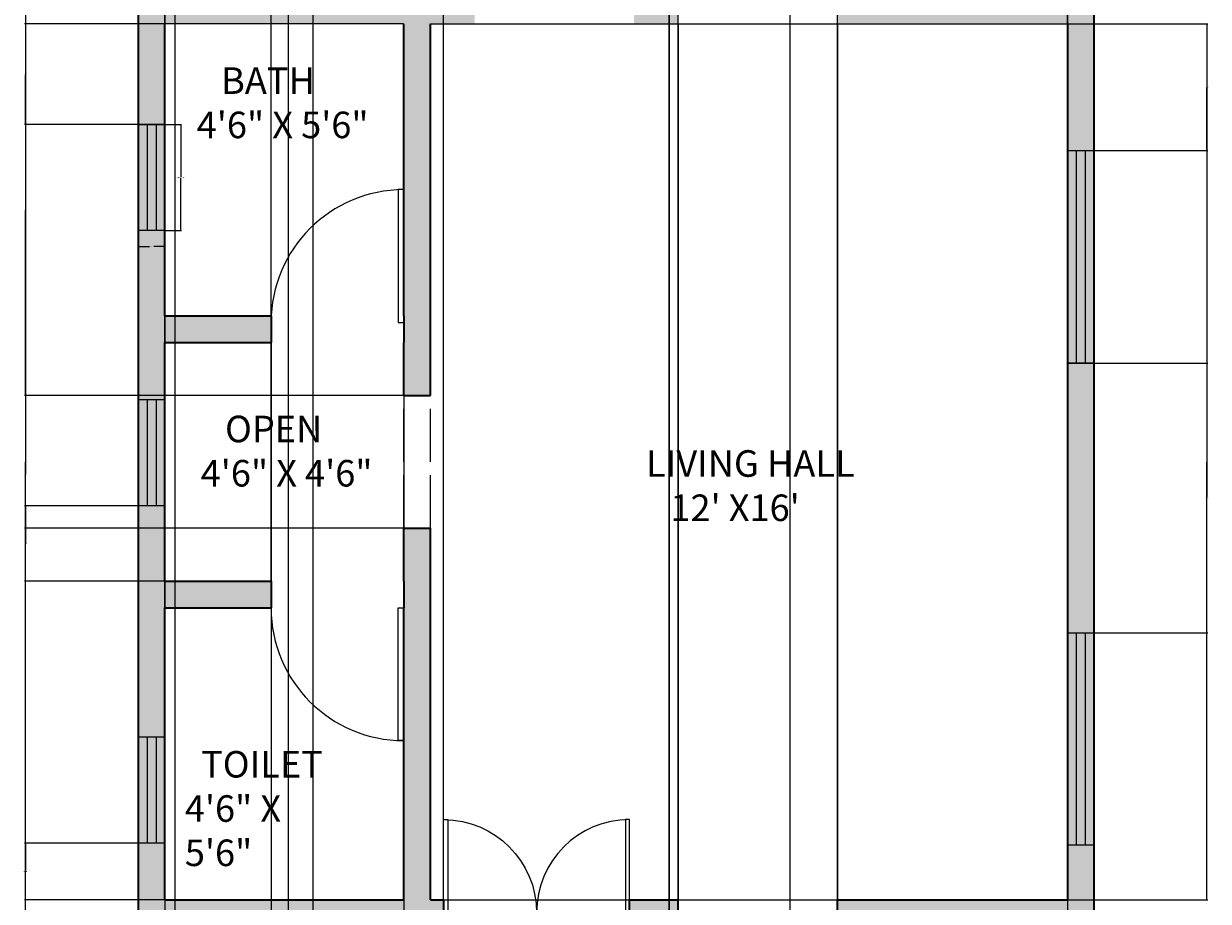
# Model space of a CAD drawing. Units: feet. Extents: x 4596233 to 4596501, y 5666486 to 5667044.
# Tile 2 of 3: x 4596233 to 4596501, y 5666688 to 5666886. Entities that reach past the tile are written whole.
import ezdxf

# ---------------------------------------------------------------- set-up
doc = ezdxf.new("R2010")
doc.units = ezdxf.units.FT
doc.linetypes.add('ACAD_ISO02W100', pattern=[15, 12, -3])
for name, color, linetype, lineweight in [('A-ANNO-DIMS', 2, 'Continuous', 18), ('A-DOOR-OVHD', 240, 'ACAD_ISO02W100', 18), ('A-WALL', 7, 'Continuous', 35), ('ANNOTATION', 170, 'Continuous', 18), ('DOOR', 240, 'Continuous', 18)]:
    doc.layers.add(name, color=color, linetype=linetype, lineweight=lineweight)
doc.layers.add('A-GLAZ', color=2, linetype='Continuous', lineweight=18, true_color=0xf1eb1f)
doc.layers.add('A-WALL-PATT', color=251, linetype='Continuous', lineweight=13, true_color=0x636466)
doc.styles.get("Standard").update_dxf_attribs({"font": 'arial.ttf'})
doc.dimstyles.get("Standard").update_dxf_attribs({"dimtxt": 0.18, "dimasz": 0.18, "dimexe": 0.18, "dimexo": 0.0625, "dimgap": 0.09, "dimtad": 0, "dimtih": 1, "dimtoh": 1, "dimdec": 0, "dimzin": 0, "dimdsep": 46, "dimlunit": 3, "dimtxsty": 'Standard', "dimcen": 0.09, "dimadec": 0, "dimazin": 0, "dimtfac": 1, "dimtdec": 0, "dimtofl": 0, "dimtmove": 0, "dimatfit": 3, "dimfxl": 1, "dimtolj": 1, "dimtzin": 0, "dimarcsym": 0})

# ---------------------------------------------------------------- blocks, each defined once
blk = doc.blocks.new('*U3')
for p, q in [((0, 0), (0, -6)), ((-40, 0), (-40, -6))]:
    blk.add_line(p, q)
blk.add_lwpolyline([(0, 0), (0, 40), (-1.75, 40), (-1.75, 0)], close=True)
blk.add_arc((0, 0), 40, 90, 180)
blk = doc.blocks.new('*U2')
for p, q in [((-40, 0), (-40, 6)), ((0, 0), (0, 6))]:
    blk.add_line(p, q)
blk.add_lwpolyline([(0, 0), (0, -40), (-1.75, -40), (-1.75, 0)], close=True)
blk.add_arc((0, 0), 40, 180, 270)
blk = doc.blocks.new('WIN-48IN')
h = blk.add_hatch(color=256)
h.dxf.hatch_style = 1
h.paths.add_polyline_path([(48, 2), (48, 4), (0, 4), (0, 2)])
for p, q in [((0, 6), (48, 6)), ((0, 0), (0, 6)), ((48, 6), (48, 0)), ((0, 4), (48, 4)), ((0, 2), (48, 2)), ((48, 0), (0, 0))]:
    blk.add_line(p, q)
blk = doc.blocks.new('WIN-24IN')
h = blk.add_hatch(color=256)
h.dxf.hatch_style = 1
h.paths.add_polyline_path([(2, 0), (4, 0), (4, 24), (2, 24)])
for p, q in [((0, 0), (0, 24)), ((0, 24), (6, 24)), ((2, 24), (2, 0)), ((4, 24), (4, 0)), ((6, 24), (6, 0)), ((6, 0), (0, 0))]:
    blk.add_line(p, q)
blk = doc.blocks.new('*D9')
at = {"layer": 'A-ANNO-DIMS', "color": 0, "lineweight": -2, "transparency": 16777216}
for p, q in [((4596264.91, 5666863.39), (4596268.63, 5666863.39)), ((4596268.45, 5666863.21), (4596268.45, 5666851.57)), ((4596268.45, 5666839.57), (4596268.45, 5666851.21)), ((4596264.91, 5666839.39), (4596268.63, 5666839.39))]:
    blk.add_line(p, q, dxfattribs=at)
at = {"layer": 'A-ANNO-DIMS', "color": 0, "transparency": 16777216}
for points in [[(4596268.42, 5666863.21), (4596268.48, 5666863.21), (4596268.45, 5666863.39)], [(4596268.42, 5666839.57), (4596268.48, 5666839.57), (4596268.45, 5666839.39)]]:
    blk.add_solid(points, dxfattribs=at)
at = {"layer": 'Defpoints', "color": 0, "transparency": 16777216}
for p in [(4596264.85, 5666863.39), (4596268.45, 5666863.39), (4596264.85, 5666839.39)]:
    blk.add_point(p, dxfattribs=at)
at = {"layer": 'A-ANNO-DIMS', "color": 0, "transparency": 16777216, "insert": (4596268.45, 5666851.39), "char_height": 0.18, "attachment_point": 5}
blk.add_mtext('\\A1;WINDOW 24 TYP.', dxfattribs=at)
blk = doc.blocks.new('*D10')
at = {"layer": 'A-ANNO-DIMS', "color": 0, "lineweight": -2, "transparency": 16777216}
for p, q in [((4596258.85, 5666839.33), (4596258.85, 5666835.61)), ((4596264.85, 5666839.33), (4596264.85, 5666835.61)), ((4596259.03, 5666835.79), (4596261.39, 5666835.79)), ((4596264.67, 5666835.79), (4596262.31, 5666835.79))]:
    blk.add_line(p, q, dxfattribs=at)
at = {"layer": 'A-ANNO-DIMS', "color": 0, "transparency": 16777216}
for points in [[(4596259.03, 5666835.82), (4596259.03, 5666835.76), (4596258.85, 5666835.79)], [(4596264.67, 5666835.82), (4596264.67, 5666835.76), (4596264.85, 5666835.79)]]:
    blk.add_solid(points, dxfattribs=at)
at = {"layer": 'Defpoints', "color": 0, "transparency": 16777216}
for p in [(4596258.85, 5666839.39), (4596264.85, 5666839.39), (4596264.85, 5666835.79)]:
    blk.add_point(p, dxfattribs=at)
at = {"layer": 'A-ANNO-DIMS', "color": 0, "transparency": 16777216, "insert": (4596261.85, 5666835.79), "char_height": 0.18, "attachment_point": 5}
blk.add_mtext('\\A1;6 TYP.', dxfattribs=at)
blk = doc.blocks.new('*D12')
at = {"layer": 'A-ANNO-DIMS', "color": 0, "lineweight": -2, "transparency": 16777216}
for p, q in [((4596258.79, 5667018.15), (4596233.12, 5667018.15)), ((4596233.3, 5667017.97), (4596233.3, 5666784.33)), ((4596233.3, 5666550.33), (4596233.3, 5666783.97)), ((4596258.79, 5666550.15), (4596233.12, 5666550.15))]:
    blk.add_line(p, q, dxfattribs=at)
at = {"layer": 'A-ANNO-DIMS', "color": 0, "transparency": 16777216}
for points in [[(4596233.27, 5667017.97), (4596233.33, 5667017.97), (4596233.3, 5667018.15)], [(4596233.27, 5666550.33), (4596233.33, 5666550.33), (4596233.3, 5666550.15)]]:
    blk.add_solid(points, dxfattribs=at)
at = {"layer": 'Defpoints', "color": 0, "transparency": 16777216}
for p in [(4596233.3, 5667018.15), (4596258.85, 5667018.15), (4596258.85, 5666550.15)]:
    blk.add_point(p, dxfattribs=at)
at = {"layer": 'A-ANNO-DIMS', "color": 0, "transparency": 16777216, "insert": (4596233.3, 5666784.15), "char_height": 0.18, "attachment_point": 5}
blk.add_mtext('\\A1;468', dxfattribs=at)
blk = doc.blocks.new('*D14')
at = {"layer": 'A-ANNO-DIMS', "color": 0, "lineweight": -2, "transparency": 16777216}
for p, q in [((4596324.91, 5666886.15), (4596500.58, 5666886.15)), ((4596500.4, 5666885.97), (4596500.4, 5666787.33)), ((4596500.4, 5666688.33), (4596500.4, 5666786.97)), ((4596324.91, 5666688.15), (4596500.58, 5666688.15))]:
    blk.add_line(p, q, dxfattribs=at)
at = {"layer": 'A-ANNO-DIMS', "color": 0, "transparency": 16777216}
for points in [[(4596500.37, 5666885.97), (4596500.43, 5666885.97), (4596500.4, 5666886.15)], [(4596500.37, 5666688.33), (4596500.43, 5666688.33), (4596500.4, 5666688.15)]]:
    blk.add_solid(points, dxfattribs=at)
at = {"layer": 'Defpoints', "color": 0, "transparency": 16777216}
for p in [(4596324.85, 5666886.15), (4596500.4, 5666886.15), (4596324.85, 5666688.15)]:
    blk.add_point(p, dxfattribs=at)
at = {"layer": 'A-ANNO-DIMS', "color": 0, "transparency": 16777216, "insert": (4596500.4, 5666787.15), "char_height": 0.18, "attachment_point": 5}
blk.add_mtext('\\A1;198', dxfattribs=at)
blk = doc.blocks.new('*D15')
at = {"layer": 'A-ANNO-DIMS', "color": 0, "lineweight": -2, "transparency": 16777216}
for p, q in [((4596378.85, 5666964.09), (4596378.85, 5666485.84)), ((4596468.85, 5666964.09), (4596468.85, 5666485.84)), ((4596379.03, 5666486.02), (4596423.63, 5666486.02)), ((4596468.67, 5666486.02), (4596424.07, 5666486.02))]:
    blk.add_line(p, q, dxfattribs=at)
at = {"layer": 'A-ANNO-DIMS', "color": 0, "transparency": 16777216}
for points in [[(4596379.03, 5666486.05), (4596379.03, 5666485.99), (4596378.85, 5666486.02)], [(4596468.67, 5666486.05), (4596468.67, 5666485.99), (4596468.85, 5666486.02)]]:
    blk.add_solid(points, dxfattribs=at)
at = {"layer": 'Defpoints', "color": 0, "transparency": 16777216}
for p in [(4596378.85, 5666964.15), (4596468.85, 5666964.15), (4596468.85, 5666486.02)]:
    blk.add_point(p, dxfattribs=at)
at = {"layer": 'A-ANNO-DIMS', "color": 0, "transparency": 16777216, "insert": (4596423.85, 5666486.02), "char_height": 0.18, "attachment_point": 5}
blk.add_mtext('\\A1;90', dxfattribs=at)
blk = doc.blocks.new('*D17')
at = {"layer": 'A-ANNO-DIMS', "color": 0, "lineweight": -2, "transparency": 16777216}
for p, q in [((4596380.85, 5666688.21), (4596380.85, 5667043.88)), ((4596381.03, 5667043.7), (4596398.63, 5667043.7)), ((4596416.67, 5667043.7), (4596399.07, 5667043.7)), ((4596416.85, 5666688.21), (4596416.85, 5667043.88))]:
    blk.add_line(p, q, dxfattribs=at)
at = {"layer": 'A-ANNO-DIMS', "color": 0, "transparency": 16777216}
for points in [[(4596381.03, 5667043.73), (4596381.03, 5667043.67), (4596380.85, 5667043.7)], [(4596416.67, 5667043.73), (4596416.67, 5667043.67), (4596416.85, 5667043.7)]]:
    blk.add_solid(points, dxfattribs=at)
at = {"layer": 'Defpoints', "color": 0, "transparency": 16777216}
for p in [(4596416.85, 5667043.7), (4596380.85, 5666688.15), (4596416.85, 5666688.15)]:
    blk.add_point(p, dxfattribs=at)
at = {"layer": 'A-ANNO-DIMS', "color": 0, "transparency": 16777216, "insert": (4596398.85, 5667043.7), "char_height": 0.18, "attachment_point": 5}
blk.add_mtext('\\A1;36', dxfattribs=at)
blk = doc.blocks.new('*D18')
at = {"layer": 'A-ANNO-DIMS', "color": 0, "lineweight": -2, "transparency": 16777216}
for p, q in [((4596288.85, 5666814.09), (4596288.85, 5666485.84)), ((4596318.85, 5666814.09), (4596318.85, 5666485.84)), ((4596289.03, 5666486.02), (4596303.63, 5666486.02)), ((4596318.67, 5666486.02), (4596304.07, 5666486.02))]:
    blk.add_line(p, q, dxfattribs=at)
at = {"layer": 'A-ANNO-DIMS', "color": 0, "transparency": 16777216}
for points in [[(4596289.03, 5666486.05), (4596289.03, 5666485.99), (4596288.85, 5666486.02)], [(4596318.67, 5666486.05), (4596318.67, 5666485.99), (4596318.85, 5666486.02)]]:
    blk.add_solid(points, dxfattribs=at)
at = {"layer": 'Defpoints', "color": 0, "transparency": 16777216}
for p in [(4596288.85, 5666814.15), (4596318.85, 5666814.15), (4596318.85, 5666486.02)]:
    blk.add_point(p, dxfattribs=at)
at = {"layer": 'A-ANNO-DIMS', "color": 0, "transparency": 16777216, "insert": (4596303.85, 5666486.02), "char_height": 0.18, "attachment_point": 5}
blk.add_mtext('\\A1;30', dxfattribs=at)
blk = doc.blocks.new('*D19')
at = {"layer": 'A-ANNO-DIMS', "color": 0, "lineweight": -2, "transparency": 16777216}
for p, q in [((4596318.79, 5666802.15), (4596233.12, 5666802.15)), ((4596233.3, 5666801.97), (4596233.3, 5666787.33)), ((4596233.3, 5666772.33), (4596233.3, 5666786.97)), ((4596318.79, 5666772.15), (4596233.12, 5666772.15))]:
    blk.add_line(p, q, dxfattribs=at)
at = {"layer": 'A-ANNO-DIMS', "color": 0, "transparency": 16777216}
for points in [[(4596233.27, 5666801.97), (4596233.33, 5666801.97), (4596233.3, 5666802.15)], [(4596233.27, 5666772.33), (4596233.33, 5666772.33), (4596233.3, 5666772.15)]]:
    blk.add_solid(points, dxfattribs=at)
at = {"layer": 'Defpoints', "color": 0, "transparency": 16777216}
for p in [(4596233.3, 5666802.15), (4596318.85, 5666802.15), (4596318.85, 5666772.15)]:
    blk.add_point(p, dxfattribs=at)
at = {"layer": 'A-ANNO-DIMS', "color": 0, "transparency": 16777216, "insert": (4596233.3, 5666787.15), "char_height": 0.18, "attachment_point": 5}
blk.add_mtext('\\A1;30', dxfattribs=at)
blk = doc.blocks.new('*D21')
at = {"layer": 'A-ANNO-DIMS', "color": 0, "lineweight": -2, "transparency": 16777216}
for p, q in [((4596380.85, 5666886.09), (4596380.85, 5666485.84)), ((4596416.85, 5666886.09), (4596416.85, 5666485.84)), ((4596381.03, 5666486.02), (4596398.63, 5666486.02)), ((4596416.67, 5666486.02), (4596399.07, 5666486.02))]:
    blk.add_line(p, q, dxfattribs=at)
at = {"layer": 'A-ANNO-DIMS', "color": 0, "transparency": 16777216}
for points in [[(4596381.03, 5666486.05), (4596381.03, 5666485.99), (4596380.85, 5666486.02)], [(4596416.67, 5666486.05), (4596416.67, 5666485.99), (4596416.85, 5666486.02)]]:
    blk.add_solid(points, dxfattribs=at)
at = {"layer": 'Defpoints', "color": 0, "transparency": 16777216}
for p in [(4596380.85, 5666886.15), (4596416.85, 5666886.15), (4596416.85, 5666486.02)]:
    blk.add_point(p, dxfattribs=at)
at = {"layer": 'A-ANNO-DIMS', "color": 0, "transparency": 16777216, "insert": (4596398.85, 5666486.02), "char_height": 0.18, "attachment_point": 5}
blk.add_mtext('\\A1;36', dxfattribs=at)
blk = doc.blocks.new('*D22')
at = {"layer": 'A-ANNO-DIMS', "color": 0, "lineweight": -2, "transparency": 16777216}
for p, q in [((4596264.85, 5667012.09), (4596264.85, 5666485.84)), ((4596292.72, 5667012.09), (4596292.72, 5666485.84)), ((4596265.03, 5666486.02), (4596278.39, 5666486.02)), ((4596292.54, 5666486.02), (4596279.18, 5666486.02))]:
    blk.add_line(p, q, dxfattribs=at)
at = {"layer": 'A-ANNO-DIMS', "color": 0, "transparency": 16777216}
for points in [[(4596265.03, 5666486.05), (4596265.03, 5666485.99), (4596264.85, 5666486.02)], [(4596292.54, 5666486.05), (4596292.54, 5666485.99), (4596292.72, 5666486.02)]]:
    blk.add_solid(points, dxfattribs=at)
at = {"layer": 'Defpoints', "color": 0, "transparency": 16777216}
for p in [(4596264.85, 5667012.15), (4596292.72, 5667012.15), (4596292.72, 5666486.02)]:
    blk.add_point(p, dxfattribs=at)
at = {"layer": 'A-ANNO-DIMS', "color": 0, "transparency": 16777216, "insert": (4596278.78, 5666486.02), "char_height": 0.18, "attachment_point": 5}
blk.add_mtext('\\A1;27.87', dxfattribs=at)
blk = doc.blocks.new('*D25')
at = {"layer": 'A-ANNO-DIMS', "color": 0, "lineweight": -2, "transparency": 16777216}
for p, q in [((4596468.91, 5666886.15), (4596500.58, 5666886.15)), ((4596500.4, 5666885.97), (4596500.4, 5666871.99)), ((4596500.4, 5666857.65), (4596500.4, 5666871.63)), ((4596468.91, 5666857.47), (4596500.58, 5666857.47))]:
    blk.add_line(p, q, dxfattribs=at)
at = {"layer": 'A-ANNO-DIMS', "color": 0, "transparency": 16777216}
for points in [[(4596500.37, 5666885.97), (4596500.43, 5666885.97), (4596500.4, 5666886.15)], [(4596500.37, 5666857.65), (4596500.43, 5666857.65), (4596500.4, 5666857.47)]]:
    blk.add_solid(points, dxfattribs=at)
at = {"layer": 'Defpoints', "color": 0, "transparency": 16777216}
for p in [(4596468.85, 5666886.15), (4596500.4, 5666886.15), (4596468.85, 5666857.47)]:
    blk.add_point(p, dxfattribs=at)
at = {"layer": 'A-ANNO-DIMS', "color": 0, "transparency": 16777216, "insert": (4596500.4, 5666871.81), "char_height": 0.18, "attachment_point": 5}
blk.add_mtext('\\A1;28.68', dxfattribs=at)
blk = doc.blocks.new('*D26')
at = {"layer": 'A-ANNO-DIMS', "color": 0, "lineweight": -2, "transparency": 16777216}
for p, q in [((4596468.91, 5666809.47), (4596500.58, 5666809.47)), ((4596500.4, 5666809.29), (4596500.4, 5666779.18)), ((4596500.4, 5666748.71), (4596500.4, 5666778.82)), ((4596468.91, 5666748.53), (4596500.58, 5666748.53))]:
    blk.add_line(p, q, dxfattribs=at)
at = {"layer": 'A-ANNO-DIMS', "color": 0, "transparency": 16777216}
for points in [[(4596500.37, 5666809.29), (4596500.43, 5666809.29), (4596500.4, 5666809.47)], [(4596500.37, 5666748.71), (4596500.43, 5666748.71), (4596500.4, 5666748.53)]]:
    blk.add_solid(points, dxfattribs=at)
at = {"layer": 'Defpoints', "color": 0, "transparency": 16777216}
for p in [(4596468.85, 5666809.47), (4596500.4, 5666809.47), (4596468.85, 5666748.53)]:
    blk.add_point(p, dxfattribs=at)
at = {"layer": 'A-ANNO-DIMS', "color": 0, "transparency": 16777216, "insert": (4596500.4, 5666779), "char_height": 0.18, "attachment_point": 5}
blk.add_mtext('\\A1;60.93', dxfattribs=at)
blk = doc.blocks.new('*D28')
at = {"layer": 'A-ANNO-DIMS', "color": 0, "lineweight": -2, "transparency": 16777216}
for p, q in [((4596378.85, 5666556.21), (4596378.85, 5667043.88)), ((4596379.03, 5667043.7), (4596392.04, 5667043.7)), ((4596405.99, 5667043.7), (4596392.97, 5667043.7)), ((4596406.17, 5666556.21), (4596406.17, 5667043.88))]:
    blk.add_line(p, q, dxfattribs=at)
at = {"layer": 'A-ANNO-DIMS', "color": 0, "transparency": 16777216}
for points in [[(4596379.03, 5667043.73), (4596379.03, 5667043.67), (4596378.85, 5667043.7)], [(4596405.99, 5667043.73), (4596405.99, 5667043.67), (4596406.17, 5667043.7)]]:
    blk.add_solid(points, dxfattribs=at)
at = {"layer": 'Defpoints', "color": 0, "transparency": 16777216}
for p in [(4596406.17, 5667043.7), (4596378.85, 5666556.15), (4596406.17, 5666556.15)]:
    blk.add_point(p, dxfattribs=at)
at = {"layer": 'A-ANNO-DIMS', "color": 0, "transparency": 16777216, "insert": (4596392.51, 5667043.7), "char_height": 0.18, "attachment_point": 5}
blk.add_mtext('\\A1;27.317', dxfattribs=at)
blk = doc.blocks.new('*D29')
at = {"layer": 'A-ANNO-DIMS', "color": 0, "lineweight": -2, "transparency": 16777216}
for p, q in [((4596258.79, 5666701.02), (4596233.12, 5666701.02)), ((4596233.3, 5666700.84), (4596233.3, 5666694.77)), ((4596233.3, 5666688.33), (4596233.3, 5666694.4)), ((4596264.79, 5666688.15), (4596233.12, 5666688.15))]:
    blk.add_line(p, q, dxfattribs=at)
at = {"layer": 'A-ANNO-DIMS', "color": 0, "transparency": 16777216}
for points in [[(4596233.27, 5666700.84), (4596233.33, 5666700.84), (4596233.3, 5666701.02)], [(4596233.27, 5666688.33), (4596233.33, 5666688.33), (4596233.3, 5666688.15)]]:
    blk.add_solid(points, dxfattribs=at)
at = {"layer": 'Defpoints', "color": 0, "transparency": 16777216}
for p in [(4596233.3, 5666701.02), (4596258.85, 5666701.02), (4596264.85, 5666688.15)]:
    blk.add_point(p, dxfattribs=at)
at = {"layer": 'A-ANNO-DIMS', "color": 0, "transparency": 16777216, "insert": (4596233.3, 5666694.58), "char_height": 0.18, "attachment_point": 5}
blk.add_mtext('\\A1;12.872', dxfattribs=at)
blk = doc.blocks.new('*D30')
at = {"layer": 'A-ANNO-DIMS', "color": 0, "lineweight": -2, "transparency": 16777216}
for p, q in [((4596264.79, 5666777.21), (4596233.12, 5666777.21)), ((4596233.3, 5666777.03), (4596233.3, 5666768.86)), ((4596233.3, 5666760.33), (4596233.3, 5666768.5)), ((4596264.79, 5666760.15), (4596233.12, 5666760.15))]:
    blk.add_line(p, q, dxfattribs=at)
at = {"layer": 'A-ANNO-DIMS', "color": 0, "transparency": 16777216}
for points in [[(4596233.27, 5666777.03), (4596233.33, 5666777.03), (4596233.3, 5666777.21)], [(4596233.27, 5666760.33), (4596233.33, 5666760.33), (4596233.3, 5666760.15)]]:
    blk.add_solid(points, dxfattribs=at)
at = {"layer": 'Defpoints', "color": 0, "transparency": 16777216}
for p in [(4596233.3, 5666777.21), (4596264.85, 5666777.21), (4596264.85, 5666760.15)]:
    blk.add_point(p, dxfattribs=at)
at = {"layer": 'A-ANNO-DIMS', "color": 0, "transparency": 16777216, "insert": (4596233.3, 5666768.68), "char_height": 0.18, "attachment_point": 5}
blk.add_mtext('\\A1;17.063', dxfattribs=at)
blk = doc.blocks.new('*D31')
at = {"layer": 'A-ANNO-DIMS', "color": 0, "lineweight": -2, "transparency": 16777216}
for p, q in [((4596264.79, 5666886.15), (4596233.12, 5666886.15)), ((4596233.3, 5666885.97), (4596233.3, 5666874.95)), ((4596233.3, 5666863.57), (4596233.3, 5666874.59)), ((4596264.79, 5666863.39), (4596233.12, 5666863.39))]:
    blk.add_line(p, q, dxfattribs=at)
at = {"layer": 'A-ANNO-DIMS', "color": 0, "transparency": 16777216}
for points in [[(4596233.27, 5666885.97), (4596233.33, 5666885.97), (4596233.3, 5666886.15)], [(4596233.27, 5666863.57), (4596233.33, 5666863.57), (4596233.3, 5666863.39)]]:
    blk.add_solid(points, dxfattribs=at)
at = {"layer": 'Defpoints', "color": 0, "transparency": 16777216}
for p in [(4596233.3, 5666886.15), (4596264.85, 5666886.15), (4596264.85, 5666863.39)]:
    blk.add_point(p, dxfattribs=at)
at = {"layer": 'A-ANNO-DIMS', "color": 0, "transparency": 16777216, "insert": (4596233.3, 5666874.77), "char_height": 0.18, "attachment_point": 5}
blk.add_mtext('\\A1;22.757', dxfattribs=at)
blk = doc.blocks.new('*D33')
at = {"layer": 'A-ANNO-DIMS', "color": 0, "lineweight": -2, "transparency": 16777216}
for p, q in [((4596267.15, 5666650.02), (4596267.15, 5667043.88)), ((4596267.33, 5667043.7), (4596282.36, 5667043.7)), ((4596298.17, 5667043.7), (4596283.14, 5667043.7)), ((4596298.35, 5666650.02), (4596298.35, 5667043.88))]:
    blk.add_line(p, q, dxfattribs=at)
at = {"layer": 'A-ANNO-DIMS', "color": 0, "transparency": 16777216}
for points in [[(4596267.33, 5667043.73), (4596267.33, 5667043.67), (4596267.15, 5667043.7)], [(4596298.17, 5667043.73), (4596298.17, 5667043.67), (4596298.35, 5667043.7)]]:
    blk.add_solid(points, dxfattribs=at)
at = {"layer": 'Defpoints', "color": 0, "transparency": 16777216}
for p in [(4596298.35, 5667043.7), (4596267.15, 5666649.96), (4596298.35, 5666649.96)]:
    blk.add_point(p, dxfattribs=at)
at = {"layer": 'A-ANNO-DIMS', "color": 0, "transparency": 16777216, "insert": (4596282.75, 5667043.7), "char_height": 0.18, "attachment_point": 5}
blk.add_mtext('\\A1;31.19', dxfattribs=at)
blk = doc.blocks.new('*D35')
at = {"layer": 'A-ANNO-DIMS', "color": 0, "lineweight": -2, "transparency": 16777216}
for p, q in [((4596416.85, 5666688.21), (4596416.85, 5667043.88)), ((4596417.03, 5667043.7), (4596442.63, 5667043.7)), ((4596468.67, 5667043.7), (4596443.07, 5667043.7)), ((4596468.85, 5666688.21), (4596468.85, 5667043.88))]:
    blk.add_line(p, q, dxfattribs=at)
at = {"layer": 'A-ANNO-DIMS', "color": 0, "transparency": 16777216}
for points in [[(4596417.03, 5667043.73), (4596417.03, 5667043.67), (4596416.85, 5667043.7)], [(4596468.67, 5667043.73), (4596468.67, 5667043.67), (4596468.85, 5667043.7)]]:
    blk.add_solid(points, dxfattribs=at)
at = {"layer": 'Defpoints', "color": 0, "transparency": 16777216}
for p in [(4596468.85, 5667043.7), (4596416.85, 5666688.15), (4596468.85, 5666688.15)]:
    blk.add_point(p, dxfattribs=at)
at = {"layer": 'A-ANNO-DIMS', "color": 0, "transparency": 16777216, "insert": (4596442.85, 5667043.7), "char_height": 0.18, "attachment_point": 5}
blk.add_mtext('\\A1;52', dxfattribs=at)
blk = doc.blocks.new('*D36')
at = {"layer": 'A-ANNO-DIMS', "color": 0, "lineweight": -2, "transparency": 16777216}
for p, q in [((4596318.79, 5666886.15), (4596233.12, 5666886.15)), ((4596233.3, 5666885.97), (4596233.3, 5666844.33)), ((4596233.3, 5666802.33), (4596233.3, 5666843.97)), ((4596318.79, 5666802.15), (4596233.12, 5666802.15))]:
    blk.add_line(p, q, dxfattribs=at)
at = {"layer": 'A-ANNO-DIMS', "color": 0, "transparency": 16777216}
for points in [[(4596233.27, 5666885.97), (4596233.33, 5666885.97), (4596233.3, 5666886.15)], [(4596233.27, 5666802.33), (4596233.33, 5666802.33), (4596233.3, 5666802.15)]]:
    blk.add_solid(points, dxfattribs=at)
at = {"layer": 'Defpoints', "color": 0, "transparency": 16777216}
for p in [(4596233.3, 5666886.15), (4596318.85, 5666886.15), (4596318.85, 5666802.15)]:
    blk.add_point(p, dxfattribs=at)
at = {"layer": 'A-ANNO-DIMS', "color": 0, "transparency": 16777216, "insert": (4596233.3, 5666844.15), "char_height": 0.18, "attachment_point": 5}
blk.add_mtext('\\A1;84', dxfattribs=at)
blk = doc.blocks.new('*D37')
at = {"layer": 'A-ANNO-DIMS', "color": 0, "lineweight": -2, "transparency": 16777216}
for p, q in [((4596264.85, 5666688.21), (4596264.85, 5667043.88)), ((4596265.03, 5667043.7), (4596296.13, 5667043.7)), ((4596327.67, 5667043.7), (4596296.57, 5667043.7)), ((4596327.85, 5666688.21), (4596327.85, 5667043.88))]:
    blk.add_line(p, q, dxfattribs=at)
at = {"layer": 'A-ANNO-DIMS', "color": 0, "transparency": 16777216}
for points in [[(4596265.03, 5667043.73), (4596265.03, 5667043.67), (4596264.85, 5667043.7)], [(4596327.67, 5667043.73), (4596327.67, 5667043.67), (4596327.85, 5667043.7)]]:
    blk.add_solid(points, dxfattribs=at)
at = {"layer": 'Defpoints', "color": 0, "transparency": 16777216}
for p in [(4596327.85, 5667043.7), (4596264.85, 5666688.15), (4596327.85, 5666688.15)]:
    blk.add_point(p, dxfattribs=at)
at = {"layer": 'A-ANNO-DIMS', "color": 0, "transparency": 16777216, "insert": (4596296.35, 5667043.7), "char_height": 0.18, "attachment_point": 5}
blk.add_mtext('\\A1;63', dxfattribs=at)
blk = doc.blocks.new('*D38')
at = {"layer": 'A-ANNO-DIMS', "color": 0, "lineweight": -2, "transparency": 16777216}
for p, q in [((4596416.85, 5666886.09), (4596416.85, 5666485.84)), ((4596468.85, 5666886.09), (4596468.85, 5666485.84)), ((4596417.03, 5666486.02), (4596442.63, 5666486.02)), ((4596468.67, 5666486.02), (4596443.07, 5666486.02))]:
    blk.add_line(p, q, dxfattribs=at)
at = {"layer": 'A-ANNO-DIMS', "color": 0, "transparency": 16777216}
for points in [[(4596417.03, 5666486.05), (4596417.03, 5666485.99), (4596416.85, 5666486.02)], [(4596468.67, 5666486.05), (4596468.67, 5666485.99), (4596468.85, 5666486.02)]]:
    blk.add_solid(points, dxfattribs=at)
at = {"layer": 'Defpoints', "color": 0, "transparency": 16777216}
for p in [(4596416.85, 5666886.15), (4596468.85, 5666886.15), (4596468.85, 5666486.02)]:
    blk.add_point(p, dxfattribs=at)
at = {"layer": 'A-ANNO-DIMS', "color": 0, "transparency": 16777216, "insert": (4596442.85, 5666486.02), "char_height": 0.18, "attachment_point": 5}
blk.add_mtext('\\A1;52', dxfattribs=at)
blk = doc.blocks.new('*D39')
at = {"layer": 'A-ANNO-DIMS', "color": 0, "lineweight": -2, "transparency": 16777216}
for p, q in [((4596264.85, 5666760.21), (4596264.85, 5667043.88)), ((4596265.03, 5667043.7), (4596276.63, 5667043.7)), ((4596288.67, 5667043.7), (4596277.07, 5667043.7)), ((4596288.85, 5666760.21), (4596288.85, 5667043.88))]:
    blk.add_line(p, q, dxfattribs=at)
at = {"layer": 'A-ANNO-DIMS', "color": 0, "transparency": 16777216}
for points in [[(4596265.03, 5667043.73), (4596265.03, 5667043.67), (4596264.85, 5667043.7)], [(4596288.67, 5667043.73), (4596288.67, 5667043.67), (4596288.85, 5667043.7)]]:
    blk.add_solid(points, dxfattribs=at)
at = {"layer": 'Defpoints', "color": 0, "transparency": 16777216}
for p in [(4596288.85, 5667043.7), (4596264.85, 5666760.15), (4596288.85, 5666760.15)]:
    blk.add_point(p, dxfattribs=at)
at = {"layer": 'A-ANNO-DIMS', "color": 0, "transparency": 16777216, "insert": (4596276.85, 5667043.7), "char_height": 0.18, "attachment_point": 5}
blk.add_mtext('\\A1;24', dxfattribs=at)

msp = doc.modelspace()

# ---------------------------------------------------------------- hatches: boundary and pattern name
at = {"layer": 'A-WALL-PATT'}
h = msp.add_hatch(color=256, dxfattribs=at)
h.dxf.hatch_style = 1
h.paths.add_polyline_path([(4596474.8511, 5667018.1479), (4596258.8511, 5667018.1479), (4596258.8511, 5666550.1479), (4596474.8511, 5666550.1479)])
h.paths.add_polyline_path([(4596372.8511, 5667012.1479), (4596372.8511, 5666892.1479), (4596370.8511, 5666892.1479), (4596370.8511, 5666891.5479), (4596370.8511, 5666886.1479), (4596380.8511, 5666886.1479), (4596380.8511, 5666892.1479), (4596378.8511, 5666892.1479), (4596378.8511, 5666964.1479), (4596380.8511, 5666964.1479), (4596380.8511, 5666970.1479), (4596378.8511, 5666970.1479), (4596378.8511, 5667012.1479), (4596468.8511, 5667012.1479), (4596468.8511, 5666970.1479), (4596416.8511, 5666970.1479), (4596416.8511, 5666964.1479), (4596468.8511, 5666964.1479), (4596468.8511, 5666892.1479), (4596416.8511, 5666892.1479), (4596416.8511, 5666886.1479), (4596468.8511, 5666886.1479), (4596468.8511, 5666688.1479), (4596416.8511, 5666688.1479), (4596416.8511, 5666682.1479), (4596468.8511, 5666682.1479), (4596468.8511, 5666556.1479), (4596378.8511, 5666556.1479), (4596378.8511, 5666682.1479), (4596380.8511, 5666682.1479), (4596380.8511, 5666687.5479), (4596380.8511, 5666688.1479), (4596369.8511, 5666688.1479), (4596369.8511, 5666685.2979), (4596369.8511, 5666682.1479), (4596372.8511, 5666682.1479), (4596372.8511, 5666556.1479), (4596264.8511, 5666556.1479), (4596264.8511, 5666682.1479), (4596327.8511, 5666682.1479), (4596327.8511, 5666685.2979), (4596327.8511, 5666688.1479), (4596324.8511, 5666688.1479), (4596324.8511, 5666772.1479), (4596318.8511, 5666772.1479), (4596318.8511, 5666760.1479), (4596318.8511, 5666754.1479), (4596318.8511, 5666724.1479), (4596318.8511, 5666688.1479), (4596264.8511, 5666688.1479), (4596264.8511, 5666754.1479), (4596288.8511, 5666754.1479), (4596288.8511, 5666758.6479), (4596288.8511, 5666760.1479), (4596264.8511, 5666760.1479), (4596264.8511, 5666814.1479), (4596288.8511, 5666814.1479), (4596288.8511, 5666818.6479), (4596288.8511, 5666820.1479), (4596264.8511, 5666820.1479), (4596264.8511, 5666886.1479), (4596318.8511, 5666886.1479), (4596318.8511, 5666820.1479), (4596318.8511, 5666818.6479), (4596318.8511, 5666814.1479), (4596318.8511, 5666802.1479), (4596324.8511, 5666802.1479), (4596324.8511, 5666886.1479), (4596334.8511, 5666886.1479), (4596334.8511, 5666891.5479), (4596334.8511, 5666892.1479), (4596264.8511, 5666892.1479), (4596264.8511, 5667012.1479)], flags=16)
h.paths.add_polyline_path([(4596316.6338, 5666680.1479), (4596316.6338, 5666661.9608), (4596301.036, 5666661.9608), (4596301.036, 5666589.119), (4596370.916, 5666589.119), (4596370.916, 5666558.119), (4596267.1547, 5666558.119), (4596267.1547, 5666680.1479)], flags=0)
h.paths.add_polyline_path([(4596282.7503, 5666649.9608), (4596298.3459, 5666649.9608), (4596298.3459, 5666586.4128), (4596333.2108, 5666586.4128), (4596333.2108, 5666572.6335), (4596282.7503, 5666572.6335)], flags=0)
h.paths.add_polyline_path([(4596380.8511, 5666682.1479), (4596382.4261, 5666682.1479), (4596382.4261, 5666646.1479), (4596380.8511, 5666646.1479)], flags=0)
h.paths.add_polyline_path([(4596270.4341, 5666856.9819), (4596311.4805, 5666856.9819), (4596311.4805, 5666879.3708), (4596270.4341, 5666879.3708)], flags=8)
h.paths.add_polyline_path([(4596271.3283, 5666778.1649), (4596312.3747, 5666778.1649), (4596312.3747, 5666800.5538), (4596271.3283, 5666800.5538)], flags=8)
h.paths.add_polyline_path([(4596401.0723, 5666924.3036), (4596440.8622, 5666924.3036), (4596440.8622, 5666946.6925), (4596401.0723, 5666946.6925)], flags=8)
h.paths.add_polyline_path([(4596396.1839, 5666976.1395), (4596449.4963, 5666976.1395), (4596449.4963, 5666998.5283), (4596396.1839, 5666998.5283)], flags=8)
h.paths.add_polyline_path([(4596288.0879, 5666956.0844), (4596336.7264, 5666956.0844), (4596336.7264, 5666978.4732), (4596288.0879, 5666978.4732)], flags=8)
h.paths.add_polyline_path([(4596267.7433, 5666702.4027), (4596308.7897, 5666702.4027), (4596308.7897, 5666724.7916), (4596267.7433, 5666724.7916)], flags=8)
h.paths.add_polyline_path([(4596371.4978, 5666770.3665), (4596425.2768, 5666770.3665), (4596425.2768, 5666792.7553), (4596371.4978, 5666792.7553)], flags=8)
h.paths.add_polyline_path([(4596414.2198, 5666615.8536), (4596452.2908, 5666615.8536), (4596452.2908, 5666638.2424), (4596414.2198, 5666638.2424)], flags=8)
h.paths.add_polyline_path([(4596310.1554, 5666620.3865), (4596350.8825, 5666620.3865), (4596350.8825, 5666642.7753), (4596310.1554, 5666642.7753)], flags=8)
h = msp.add_hatch(color=256, dxfattribs=at)
h.dxf.hatch_style = 1
h.paths.add_polyline_path([(4596474.8511, 5667018.1479), (4596258.8511, 5667018.1479), (4596258.8511, 5666550.1479), (4596474.8511, 5666550.1479)])
h.paths.add_polyline_path([(4596468.8511, 5666970.1479), (4596416.8511, 5666970.1479), (4596416.8511, 5666964.1479), (4596468.8511, 5666964.1479), (4596468.8511, 5666892.1479), (4596416.8511, 5666892.1479), (4596416.8511, 5666886.1479), (4596468.8511, 5666886.1479), (4596468.8511, 5666688.1479), (4596416.8511, 5666688.1479), (4596416.8511, 5666682.1479), (4596468.8511, 5666682.1479), (4596468.8511, 5666556.1479), (4596378.8511, 5666556.1479), (4596378.8511, 5666682.1479), (4596380.8511, 5666682.1479), (4596380.8511, 5666687.5479), (4596380.8511, 5666688.1479), (4596369.8511, 5666688.1479), (4596369.8511, 5666685.2979), (4596369.8511, 5666682.1479), (4596372.8511, 5666682.1479), (4596372.8511, 5666556.1479), (4596264.8511, 5666556.1479), (4596264.8511, 5666682.1479), (4596327.8511, 5666682.1479), (4596327.8511, 5666685.2979), (4596327.8511, 5666688.1479), (4596324.8511, 5666688.1479), (4596324.8511, 5666772.1479), (4596318.8511, 5666772.1479), (4596318.8511, 5666760.1479), (4596318.8511, 5666754.1479), (4596318.8511, 5666724.1479), (4596318.8511, 5666688.1479), (4596264.8511, 5666688.1479), (4596264.8511, 5666754.1479), (4596288.8511, 5666754.1479), (4596288.8511, 5666758.6479), (4596288.8511, 5666760.1479), (4596264.8511, 5666760.1479), (4596264.8511, 5666814.1479), (4596288.8511, 5666814.1479), (4596288.8511, 5666818.6479), (4596288.8511, 5666820.1479), (4596264.8511, 5666820.1479), (4596264.8511, 5666886.1479), (4596318.8511, 5666886.1479), (4596318.8511, 5666820.1479), (4596318.8511, 5666818.6479), (4596318.8511, 5666814.1479), (4596318.8511, 5666802.1479), (4596324.8511, 5666802.1479), (4596324.8511, 5666886.1479), (4596334.8511, 5666886.1479), (4596334.8511, 5666891.5479), (4596334.8511, 5666892.1479), (4596264.8511, 5666892.1479), (4596264.8511, 5667012.1479), (4596372.8511, 5667012.1479), (4596372.8511, 5666892.1479), (4596370.8511, 5666892.1479), (4596370.8511, 5666891.5479), (4596370.8511, 5666886.1479), (4596380.8511, 5666886.1479), (4596380.8511, 5666892.1479), (4596378.8511, 5666892.1479), (4596378.8511, 5666964.1479), (4596380.8511, 5666964.1479), (4596380.8511, 5666970.1479), (4596378.8511, 5666970.1479), (4596378.8511, 5667012.1479), (4596468.8511, 5667012.1479)], flags=16)
h.paths.add_polyline_path([(4596382.4261, 5666646.1479), (4596380.8511, 5666646.1479), (4596380.8511, 5666682.1479), (4596382.4261, 5666682.1479)], flags=0)
h.paths.add_polyline_path([(4596316.6338, 5666680.1479), (4596316.6338, 5666661.9608), (4596301.036, 5666661.9608), (4596301.036, 5666589.119), (4596370.916, 5666589.119), (4596370.916, 5666558.119), (4596267.1547, 5666558.119), (4596267.1547, 5666680.1479)], flags=0)
h.paths.add_polyline_path([(4596282.7503, 5666649.9608), (4596298.3459, 5666649.9608), (4596298.3459, 5666586.4128), (4596333.2108, 5666586.4128), (4596333.2108, 5666572.6335), (4596282.7503, 5666572.6335)], flags=0)
h.paths.add_polyline_path([(4596270.4341, 5666856.9819), (4596311.4805, 5666856.9819), (4596311.4805, 5666879.3708), (4596270.4341, 5666879.3708)], flags=8)
h.paths.add_polyline_path([(4596271.3283, 5666778.1649), (4596312.3747, 5666778.1649), (4596312.3747, 5666800.5538), (4596271.3283, 5666800.5538)], flags=8)
h.paths.add_polyline_path([(4596401.0723, 5666924.3036), (4596440.8622, 5666924.3036), (4596440.8622, 5666946.6925), (4596401.0723, 5666946.6925)], flags=8)
h.paths.add_polyline_path([(4596396.1839, 5666976.1395), (4596449.4963, 5666976.1395), (4596449.4963, 5666998.5283), (4596396.1839, 5666998.5283)], flags=8)
h.paths.add_polyline_path([(4596288.0879, 5666956.0844), (4596336.7264, 5666956.0844), (4596336.7264, 5666978.4732), (4596288.0879, 5666978.4732)], flags=8)
h.paths.add_polyline_path([(4596267.7433, 5666702.4027), (4596308.7897, 5666702.4027), (4596308.7897, 5666724.7916), (4596267.7433, 5666724.7916)], flags=8)
h.paths.add_polyline_path([(4596371.4978, 5666770.3665), (4596425.2768, 5666770.3665), (4596425.2768, 5666792.7553), (4596371.4978, 5666792.7553)], flags=8)
h.paths.add_polyline_path([(4596414.2198, 5666615.8536), (4596452.2908, 5666615.8536), (4596452.2908, 5666638.2424), (4596414.2198, 5666638.2424)], flags=8)
h.paths.add_polyline_path([(4596310.1554, 5666620.3865), (4596350.8825, 5666620.3865), (4596350.8825, 5666642.7753), (4596310.1554, 5666642.7753)], flags=8)

# ---------------------------------------------------------------- linework, layer by layer
at = {"layer": 'A-DOOR-OVHD'}
for p, q in [((4596318.8511, 5666772.1479), (4596318.8511, 5666802.1479)), ((4596324.8511, 5666772.1479), (4596324.8511, 5666802.1479))]:
    msp.add_line(p, q, dxfattribs=at)
at = {"layer": 'A-WALL'}
for p, q in [((4596258.8511, 5666550.1479), (4596258.8511, 5667018.1479)), ((4596474.8511, 5667018.1479), (4596474.8511, 5666550.1479)), ((4596264.8511, 5666820.1479), (4596264.8511, 5666886.1479)), ((4596318.8511, 5666820.1479), (4596318.8511, 5666886.1479)), ((4596324.8511, 5666802.1479), (4596324.8511, 5666886.1479)), ((4596468.8511, 5666886.1479), (4596468.8511, 5666688.1479)), ((4596264.8511, 5666820.1479), (4596288.8511, 5666820.1479)), ((4596288.8511, 5666820.1479), (4596288.8511, 5666814.1479)), ((4596318.8511, 5666820.1479), (4596318.8511, 5666814.1479)), ((4596264.8511, 5666814.1479), (4596288.8511, 5666814.1479)), ((4596264.8511, 5666760.1479), (4596264.8511, 5666814.1479)), ((4596318.8511, 5666802.1479), (4596318.8511, 5666814.1479)), ((4596318.8511, 5666802.1479), (4596324.8511, 5666802.1479)), ((4596318.8511, 5666760.1479), (4596318.8511, 5666772.1479)), ((4596318.8511, 5666772.1479), (4596324.8511, 5666772.1479)), ((4596324.8511, 5666688.1479), (4596324.8511, 5666772.1479)), ((4596264.8511, 5666760.1479), (4596288.8511, 5666760.1479)), ((4596288.8511, 5666760.1479), (4596288.8511, 5666754.1479)), ((4596318.8511, 5666760.1479), (4596318.8511, 5666754.1479)), ((4596264.8511, 5666754.1479), (4596288.8511, 5666754.1479)), ((4596264.8511, 5666688.1479), (4596264.8511, 5666754.1479)), ((4596318.8511, 5666688.1479), (4596318.8511, 5666754.1479)), ((4596264.8511, 5666688.1479), (4596318.8511, 5666688.1479)), ((4596324.8511, 5666688.1479), (4596327.8511, 5666688.1479)), ((4596327.8511, 5666688.1479), (4596327.8511, 5666682.1479)), ((4596369.8511, 5666682.1479), (4596369.8511, 5666688.1479)), ((4596369.8511, 5666688.1479), (4596380.8511, 5666688.1479)), ((4596380.8511, 5666682.1479), (4596380.8511, 5666688.1479)), ((4596416.8511, 5666682.1479), (4596416.8511, 5666688.1479)), ((4596416.8511, 5666688.1479), (4596468.8511, 5666688.1479))]:
    msp.add_line(p, q, dxfattribs=at)

# ---------------------------------------------------------------- block references
at = {"layer": 'A-GLAZ'}
for p in [(4596258.851, 5666839.3911), (4596258.851, 5666777.2107), (4596258.851, 5666701.02)]:
    msp.add_blockref('WIN-24IN', p, dxfattribs=at)
for p, rotation in [((4596468.8512, 5666857.4667), 270.0000000057113), ((4596468.8512, 5666748.5346), 270.0000000064587)]:
    msp.add_blockref('WIN-48IN', p, dxfattribs=dict(at, rotation=rotation))
at = {"layer": 'DOOR'}
for name, p, xscale, yscale, zscale in [('*U3', (4596318.8511, 5666818.6479), 0.7499999999922391, 0.7499999999922391, 0.7499999999922391), ('*U2', (4596318.8511, 5666754.1479), 0.7499999999922391, 0.7499999999922391, 0.7499999999922391), ('*U3', (4596327.8511, 5666685.2979), -0.5249999999945675, 0.5249999999945675, 0.5249999999945675), ('*U3', (4596369.8511, 5666685.2979), 0.5249999999945675, 0.5249999999945675, 0.5249999999945675)]:
    msp.add_blockref(name, p, dxfattribs=dict(at, xscale=xscale, yscale=yscale, zscale=zscale))

# ---------------------------------------------------------------- texts
at = {"layer": 'ANNOTATION', "char_height": 6, "attachment_point": 1}
for s, width, insert in [('   BATH\\P4\'6" X 5\'6"', 40.464397, (4596272.0405, 5666876.2828)), ('   OPEN\\P4\'6" X 4\'6"', 40.015786, (4596272.9347, 5666797.5722)), ("LIVING HALL\\P   12' X16'", 54.967259, (4596373.6117, 5666789.7697)), ('  TOILET\\P4\'6" X 5\'6"', 38.423604, (4596269.3497, 5666721.81))]:
    msp.add_mtext_dynamic_manual_height_columns(s, width=width, gutter_width=12.5, heights=[0], dxfattribs=dict(at, insert=insert))

# ---------------------------------------------------------------- dimensions: what is measured, and where the dimension line sits
at = {"layer": 'A-ANNO-DIMS'}
for base, p1, p2, override, picture, middle in [((4596327.8511, 5667043.6979), (4596264.8511, 5666688.1479), (4596327.8511, 5666688.1479), {"dimdec": 0, "dimlfac": 1, "dimrnd": 0, "dimzin": 0, "dimdsep": 46, "dimlunit": 2}, '*D37', (4596296.3511, 5667043.6979)), ((4596288.8511, 5667043.6979), (4596264.8511, 5666760.1479), (4596288.8511, 5666760.1479), {"dimdec": 0, "dimlfac": 1, "dimrnd": 0, "dimzin": 0, "dimdsep": 46, "dimlunit": 2}, '*D39', (4596276.8511, 5667043.6979)), ((4596298.3459, 5667043.6979), (4596267.1547, 5666649.9608), (4596298.3459, 5666649.9608), {"dimdec": 2, "dimlfac": 1, "dimrnd": 0, "dimzin": 0, "dimdsep": 46, "dimlunit": 2}, '*D33', (4596282.7503, 5667043.6979)), ((4596406.1677, 5667043.6979), (4596378.8511, 5666556.1479), (4596406.1677, 5666556.1479), {"dimdec": 3, "dimlfac": 1, "dimrnd": 0, "dimzin": 0, "dimdsep": 46, "dimlunit": 2}, '*D28', (4596392.5094, 5667043.6979)), ((4596416.8511, 5667043.6979), (4596380.8511, 5666688.1479), (4596416.8511, 5666688.1479), {"dimdec": 0, "dimlfac": 1, "dimrnd": 0, "dimzin": 0, "dimdsep": 46, "dimlunit": 2}, '*D17', (4596398.8511, 5667043.6979)), ((4596468.8511, 5667043.6979), (4596416.8511, 5666688.1479), (4596468.8511, 5666688.1479), {"dimdec": 0, "dimlfac": 1, "dimrnd": 0, "dimzin": 0, "dimdsep": 46, "dimlunit": 2}, '*D35', (4596442.8511, 5667043.6979)), ((4596292.7184, 5666486.0229), (4596264.8511, 5667012.1479), (4596292.7184, 5667012.1479), {"dimdec": 2, "dimlfac": 1, "dimrnd": 0, "dimzin": 0, "dimdsep": 46, "dimlunit": 2}, '*D22', (4596278.7847, 5666486.0229)), ((4596468.8511, 5666486.0229), (4596378.8511, 5666964.1479), (4596468.8511, 5666964.1479), {"dimdec": 0, "dimlfac": 1, "dimrnd": 0, "dimzin": 0, "dimdsep": 46, "dimlunit": 2}, '*D15', (4596423.8511, 5666486.0229)), ((4596416.8511, 5666486.0229), (4596380.8511, 5666886.1479), (4596416.8511, 5666886.1479), {"dimdec": 0, "dimlfac": 1, "dimrnd": 0, "dimzin": 0, "dimdsep": 46, "dimlunit": 2}, '*D21', (4596398.8511, 5666486.0229)), ((4596468.8511, 5666486.0229), (4596416.8511, 5666886.1479), (4596468.8511, 5666886.1479), {"dimdec": 0, "dimlfac": 1, "dimrnd": 0, "dimzin": 0, "dimdsep": 46, "dimlunit": 2}, '*D38', (4596442.8511, 5666486.0229)), ((4596318.8511, 5666486.0229), (4596288.8511, 5666814.1479), (4596318.8511, 5666814.1479), {"dimdec": 0, "dimlfac": 1, "dimrnd": 0, "dimzin": 0, "dimdsep": 46, "dimlunit": 2}, '*D18', (4596303.8511, 5666486.0229))]:
    dim = msp.add_linear_dim(base=base, p1=p1, p2=p2, dimstyle='Standard', override=override, dxfattribs=at)
    dim.commit()
    dim.dimension.update_dxf_attribs({"geometry": picture, "text_midpoint": middle})
for base, p1, p2, override, picture, middle in [((4596233.3011, 5667018.1479), (4596258.8511, 5666550.1479), (4596258.8511, 5667018.1479), {"dimdec": 0, "dimlfac": 1, "dimrnd": 0, "dimzin": 0, "dimdsep": 46, "dimlunit": 2}, '*D12', (4596233.3011, 5666784.1479)), ((4596233.3011, 5666886.1479), (4596264.8511, 5666863.3913), (4596264.8511, 5666886.1479), {"dimdec": 3, "dimlfac": 1, "dimrnd": 0, "dimzin": 0, "dimdsep": 46, "dimlunit": 2}, '*D31', (4596233.3011, 5666874.7696)), ((4596233.3011, 5666886.1479), (4596318.8511, 5666802.1479), (4596318.8511, 5666886.1479), {"dimdec": 0, "dimlfac": 1, "dimrnd": 0, "dimzin": 0, "dimdsep": 46, "dimlunit": 2}, '*D36', (4596233.3011, 5666844.1479)), ((4596500.4011, 5666886.1479), (4596324.8511, 5666688.1479), (4596324.8511, 5666886.1479), {"dimdec": 0, "dimlfac": 1, "dimrnd": 0, "dimzin": 0, "dimdsep": 46, "dimlunit": 2}, '*D14', (4596500.4011, 5666787.1479)), ((4596500.4011, 5666886.1479), (4596468.8511, 5666857.4664), (4596468.8511, 5666886.1479), {"dimdec": 2, "dimlfac": 1, "dimrnd": 0, "dimzin": 0, "dimdsep": 46, "dimlunit": 2}, '*D25', (4596500.4011, 5666871.8072)), ((4596500.4011, 5666809.4664), (4596468.8511, 5666748.5343), (4596468.8511, 5666809.4664), {"dimdec": 2, "dimlfac": 1, "dimrnd": 0, "dimzin": 0, "dimdsep": 46, "dimlunit": 2}, '*D26', (4596500.4011, 5666779.0003)), ((4596233.3011, 5666802.1479), (4596318.8511, 5666772.1479), (4596318.8511, 5666802.1479), {"dimdec": 0, "dimlfac": 1, "dimrnd": 0, "dimzin": 0, "dimdsep": 46, "dimlunit": 2}, '*D19', (4596233.3011, 5666787.1479)), ((4596233.3011, 5666777.2109), (4596264.8511, 5666760.1479), (4596264.8511, 5666777.2109), {"dimdec": 3, "dimlfac": 1, "dimrnd": 0, "dimzin": 0, "dimdsep": 46, "dimlunit": 2}, '*D30', (4596233.3011, 5666768.6794)), ((4596233.3011, 5666701.0202), (4596264.8511, 5666688.1479), (4596258.8511, 5666701.0202), {"dimdec": 3, "dimlfac": 1, "dimrnd": 0, "dimzin": 0, "dimdsep": 46, "dimlunit": 2}, '*D29', (4596233.3011, 5666694.5841))]:
    dim = msp.add_linear_dim(base=base, p1=p1, p2=p2, angle=90, dimstyle='Standard', override=override, dxfattribs=at)
    dim.commit()
    dim.dimension.update_dxf_attribs({"geometry": picture, "text_midpoint": middle})
dim = msp.add_linear_dim(base=(4596268.4511, 5666863.3913), p1=(4596264.8511, 5666839.3913), p2=(4596264.8511, 5666863.3913), angle=90, text='WINDOW <> TYP.', dimstyle='Standard', override={"dimdec": 0, "dimlfac": 1, "dimrnd": 0, "dimzin": 0, "dimdsep": 46, "dimlunit": 2}, dxfattribs=at)
dim.commit()
dim.dimension.update_dxf_attribs({"geometry": '*D9', "text_midpoint": (4596268.4511, 5666851.3913)})
dim = msp.add_linear_dim(base=(4596264.8511, 5666835.7913), p1=(4596258.8511, 5666839.3913), p2=(4596264.8511, 5666839.3913), text='<> TYP.', dimstyle='Standard', override={"dimdec": 0, "dimlfac": 1, "dimrnd": 0, "dimzin": 0, "dimdsep": 46, "dimlunit": 2}, dxfattribs=at)
dim.commit()
dim.dimension.update_dxf_attribs({"geometry": '*D10', "text_midpoint": (4596261.8511, 5666835.7913)})

doc.saveas('drawing.dxf')
